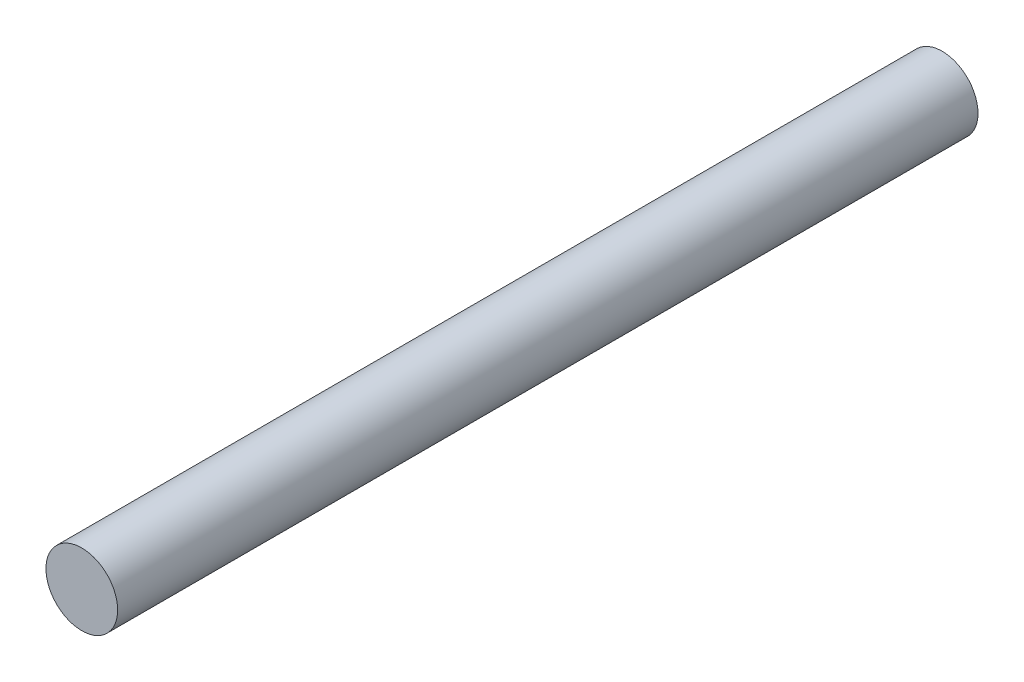
from build123d import *

# Parameters (mm, degrees)
PIN_PROFILE_6_R     = 3
PIN_BODY_6X72_DEPTH = 36


with BuildPart() as part:
    # Pin Profile Ø6 → Pin Body Ø6x72 (new, symmetric)
    with BuildSketch(Plane.XY):
        Circle(PIN_PROFILE_6_R)
    extrude(amount=PIN_BODY_6X72_DEPTH, both=True)


solid = part.part
